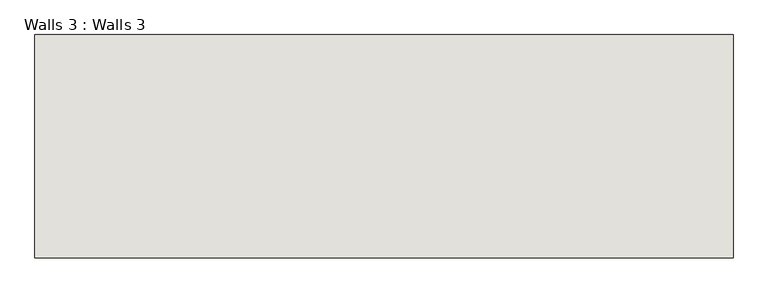
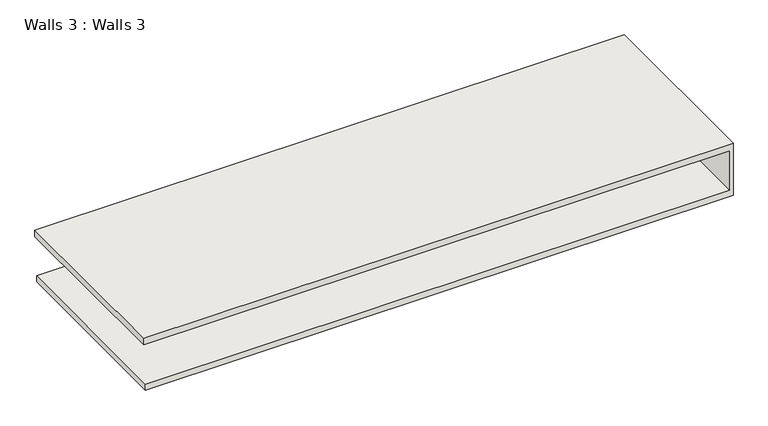
"""IFC4 building model written with IfcOpenShell, lengths in millimetres: wall geometry, Walls 3 : Walls 3."""

from ifc_helpers import new_model, si_unit, frame, origin, place, context, project, spatial, polyline, outline, extrude, source, transform, mapped, element, save


def walls_3_walls_3_546fd62f(model_context):
    return source(origin(), model_context, "Body", "SweptSolid", [
        extrude(outline(polyline([(2648.0, -18712.3660557), (2648.0, 17863.6339443), (6096.0, 17863.6339443), (6096.0, -18812.3660557), (5670.646752, -18812.3660557), (5670.646752, 17663.6339443), (3048.0, 17663.6339443), (3048.0, -18712.3660557), (2648.0, -18712.3660557)])), frame((0.0, -12737.8437646, 0.0), z_axis=(0.0, 1.0, 0.0), x_axis=(0.0, 0.0, 1.0)), (0.0, 0.0, 1.0), 11736.837277),
    ])


if __name__ == "__main__":
    model = new_model("IFC4")
    model_context = context("Model", 3, world=origin())
    ifc_project = project(units=[si_unit("LENGTHUNIT", "METRE", prefix="MILLI")], contexts=[model_context])
    site = spatial("IfcSite", under=ifc_project)
    building = spatial("IfcBuilding", under=site)
    placement = place(None, origin())
    walls_3_walls_3_shape = walls_3_walls_3_546fd62f(model_context)
    element("IfcWall", 1, ObjectType="Walls 3 : Walls 3", at=placement, inside=building, context=model_context, shape_type="MappedRepresentation", body=[
        mapped(walls_3_walls_3_shape, transform((0.0, 0.0, 0.0), x_axis=(1.0, 0.0, 0.0), y_axis=(0.0, 1.0, 0.0), z_axis=(0.0, 0.0, 1.0))),
    ])
    save(model, "model.ifc")

# Revit data of these elements
# Element 1 (IfcWall, "Walls 3 : Walls 3")
#   Materials on its faces: "Default Wall"
# Materials
#   "Default Wall": colour RGB 80 80 80, transparency 0
